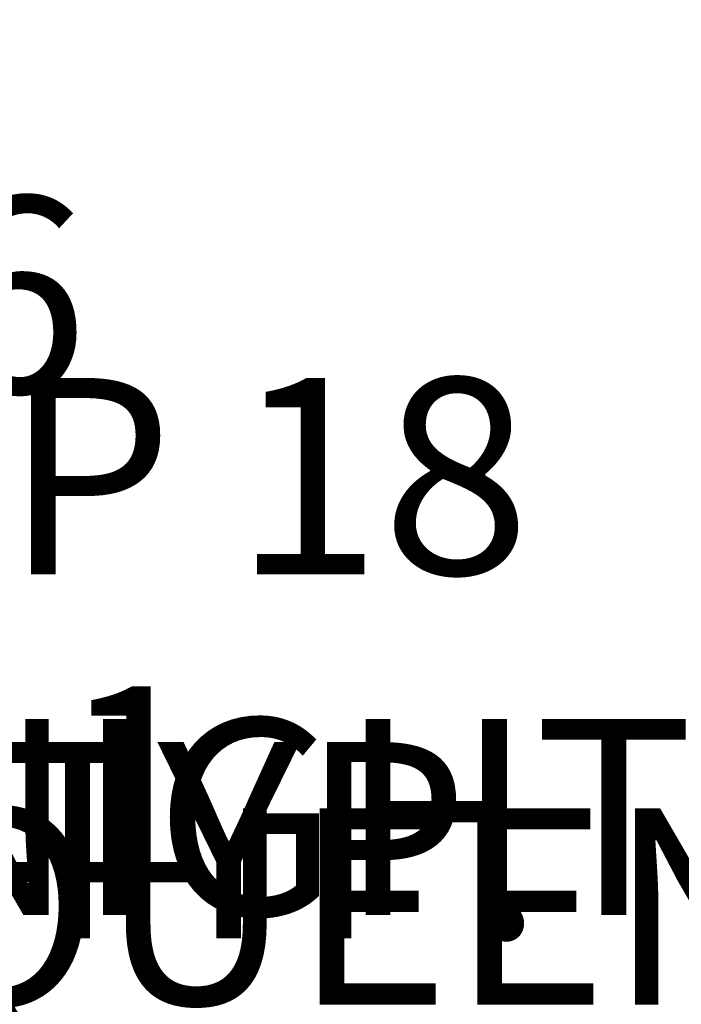
# Model space of a CAD drawing. Units: inches. Extents: x 1173 to 2157, y 515 to 1129.
# Tile 12 of 13: x 1702 to 1824, y 948 to 1129. Entities that reach past the tile are written whole.
import ezdxf

# ---------------------------------------------------------------- set-up
doc = ezdxf.new("R2010")
doc.units = ezdxf.units.IN
doc.header["$MEASUREMENT"] = 0
doc.layers.add('A-ANNO-DIMS', color=2, linetype='Continuous', lineweight=18)
doc.styles.get("Standard").update_dxf_attribs({"font": 'arial.ttf'})
doc.dimstyles.get("Standard").update_dxf_attribs({"dimtxt": 36, "dimasz": 0.18, "dimexe": 0.18, "dimexo": 0.0625, "dimgap": 0.09, "dimtad": 0, "dimtih": 1, "dimtoh": 1, "dimdec": 0, "dimrnd": 72, "dimzin": 0, "dimdsep": 46, "dimlunit": 3, "dimtxsty": 'Standard', "dimcen": 2, "dimadec": 0, "dimazin": 0, "dimtfac": 1, "dimtdec": 0, "dimtofl": 0, "dimtmove": 0, "dimatfit": 3, "dimfxl": 1, "dimtolj": 1, "dimtzin": 0, "dimarcsym": 0})

# ---------------------------------------------------------------- blocks, each defined once
blk = doc.blocks.new('*D28')
at = {"layer": 'A-ANNO-DIMS', "color": 0, "lineweight": -2, "transparency": 16777216}
for p, q in [((1581.66, 978.31), (1581.66, 966.19)), ((1661.66, 978.31), (1661.66, 966.19)), ((1581.84, 966.37), (1661.48, 966.37)), ((1661.66, 966.37), (1661.84, 966.37))]:
    blk.add_line(p, q, dxfattribs=at)
at = {"layer": 'A-ANNO-DIMS', "color": 0, "transparency": 16777216}
for points in [[(1581.84, 966.4), (1581.84, 966.34), (1581.66, 966.37)], [(1661.48, 966.4), (1661.48, 966.34), (1661.66, 966.37)]]:
    blk.add_solid(points, dxfattribs=at)
at = {"layer": 'Defpoints', "color": 0, "transparency": 16777216}
for p in [(1581.66, 978.37), (1661.66, 978.37), (1661.66, 966.37)]:
    blk.add_point(p, dxfattribs=at)
at = {"layer": 'A-ANNO-DIMS', "color": 0, "transparency": 16777216, "insert": (1904.61, 966.37), "char_height": 36, "attachment_point": 5}
blk.add_mtext('\\A1;QUEEN BED 80 TYP.', dxfattribs=at)
blk = doc.blocks.new('*D34')
at = {"layer": 'A-ANNO-DIMS', "color": 0, "lineweight": -2, "transparency": 16777216}
for p, q in [((1631.9, 978.41), (1631.9, 982.97)), ((1661.5, 978.41), (1661.5, 982.97)), ((1632.08, 982.79), (1661.32, 982.79)), ((1661.5, 982.79), (1661.68, 982.79))]:
    blk.add_line(p, q, dxfattribs=at)
at = {"layer": 'A-ANNO-DIMS', "color": 0, "transparency": 16777216}
for points in [[(1632.08, 982.82), (1632.08, 982.76), (1631.9, 982.79)], [(1661.32, 982.82), (1661.32, 982.76), (1661.5, 982.79)]]:
    blk.add_solid(points, dxfattribs=at)
at = {"layer": 'Defpoints', "color": 0, "transparency": 16777216}
for p in [(1661.5, 982.79), (1631.9, 978.35), (1661.5, 978.35)]:
    blk.add_point(p, dxfattribs=at)
at = {"layer": 'A-ANNO-DIMS', "color": 0, "transparency": 16777216, "insert": (1918.96, 982.79), "char_height": 36, "attachment_point": 5}
blk.add_mtext('\\A1;NIGHTSTAND 30 TYP.', dxfattribs=at)
blk = doc.blocks.new('*D35')
at = {"layer": 'A-ANNO-DIMS', "color": 0, "lineweight": -2, "transparency": 16777216}
for p, q in [((1631.84, 978.35), (1627.28, 978.35)), ((1627.46, 978.35), (1627.46, 978.53)), ((1627.46, 978.53), (1627.64, 978.53)), ((1627.46, 949.05), (1627.46, 978.17)), ((1631.84, 948.87), (1627.28, 948.87))]:
    blk.add_line(p, q, dxfattribs=at)
at = {"layer": 'A-ANNO-DIMS', "color": 0, "transparency": 16777216}
for points in [[(1627.43, 978.17), (1627.49, 978.17), (1627.46, 978.35)], [(1627.43, 949.05), (1627.49, 949.05), (1627.46, 948.87)]]:
    blk.add_solid(points, dxfattribs=at)
at = {"layer": 'Defpoints', "color": 0, "transparency": 16777216}
for p in [(1627.46, 978.35), (1631.9, 978.35), (1631.9, 948.87)]:
    blk.add_point(p, dxfattribs=at)
at = {"layer": 'A-ANNO-DIMS', "color": 0, "transparency": 16777216, "insert": (1715.66, 978.53), "char_height": 36, "attachment_point": 5}
blk.add_mtext('\\A1;29 TYP.', dxfattribs=at)
blk = doc.blocks.new('*D62')
at = {"layer": 'A-ANNO-DIMS', "color": 0, "lineweight": -2, "transparency": 16777216}
for p, q in [((1491.7, 1042.71), (1491.7, 1045.52)), ((1491.88, 1045.34), (1509.47, 1045.34)), ((1509.65, 1042.71), (1509.65, 1045.52)), ((1509.65, 1045.34), (1509.83, 1045.34))]:
    blk.add_line(p, q, dxfattribs=at)
at = {"layer": 'A-ANNO-DIMS', "color": 0, "transparency": 16777216}
for points in [[(1491.88, 1045.37), (1491.88, 1045.31), (1491.7, 1045.34)], [(1509.47, 1045.37), (1509.47, 1045.31), (1509.65, 1045.34)]]:
    blk.add_solid(points, dxfattribs=at)
at = {"layer": 'Defpoints', "color": 0, "transparency": 16777216}
for p in [(1509.65, 1045.34), (1491.7, 1042.65), (1509.65, 1042.65)]:
    blk.add_point(p, dxfattribs=at)
at = {"layer": 'A-ANNO-DIMS', "color": 0, "transparency": 16777216, "insert": (1657.22, 1045.34), "char_height": 36, "attachment_point": 5}
blk.add_mtext('\\A1;SINK TAP 18', dxfattribs=at)
blk = doc.blocks.new('*D90')
at = {"layer": 'A-ANNO-DIMS', "color": 0, "lineweight": -2, "transparency": 16777216}
for p, q in [((1661.73, 1044.28), (1696.15, 1044.28)), ((1695.97, 1044.1), (1695.97, 1006.94)), ((1695.97, 933.46), (1695.97, 970.62)), ((1625.73, 933.28), (1696.15, 933.28))]:
    blk.add_line(p, q, dxfattribs=at)
at = {"layer": 'A-ANNO-DIMS', "color": 0, "transparency": 16777216}
for points in [[(1695.94, 1044.1), (1696, 1044.1), (1695.97, 1044.28)], [(1695.94, 933.46), (1696, 933.46), (1695.97, 933.28)]]:
    blk.add_solid(points, dxfattribs=at)
at = {"layer": 'Defpoints', "color": 0, "transparency": 16777216}
for p in [(1661.66, 1044.28), (1625.66, 933.28), (1695.97, 933.28)]:
    blk.add_point(p, dxfattribs=at)
at = {"layer": 'A-ANNO-DIMS', "color": 0, "transparency": 16777216, "insert": (1695.97, 988.78), "char_height": 36, "attachment_point": 5}
blk.add_mtext('\\A1;111', dxfattribs=at)
blk = doc.blocks.new('*D98')
at = {"layer": 'A-ANNO-DIMS', "color": 0, "lineweight": -2, "transparency": 16777216}
for p, q in [((1625.66, 924.34), (1625.66, 1078.79)), ((1625.84, 1078.61), (1661.48, 1078.61)), ((1661.66, 924.34), (1661.66, 1078.79)), ((1661.66, 1078.61), (1661.84, 1078.61))]:
    blk.add_line(p, q, dxfattribs=at)
at = {"layer": 'A-ANNO-DIMS', "color": 0, "transparency": 16777216}
for points in [[(1625.84, 1078.64), (1625.84, 1078.58), (1625.66, 1078.61)], [(1661.48, 1078.64), (1661.48, 1078.58), (1661.66, 1078.61)]]:
    blk.add_solid(points, dxfattribs=at)
at = {"layer": 'Defpoints', "color": 0, "transparency": 16777216}
for p in [(1661.66, 1078.61), (1625.66, 924.28), (1661.66, 924.28)]:
    blk.add_point(p, dxfattribs=at)
at = {"layer": 'A-ANNO-DIMS', "color": 0, "transparency": 16777216, "insert": (1687.69, 1078.61), "char_height": 36, "attachment_point": 5}
blk.add_mtext('\\A1;36', dxfattribs=at)

msp = doc.modelspace()

# ---------------------------------------------------------------- dimensions: what is measured, and where the dimension line sits
at = {"layer": 'A-ANNO-DIMS'}
for base, p1, p2, text, picture, middle in [((1509.6463, 1045.3406), (1491.6951, 1042.6479), (1509.6463, 1042.6479), 'SINK TAP <>', '*D62', (1657.2192, 1045.3406)), ((1661.6635, 966.3712), (1581.6634, 978.3712), (1661.6635, 978.3712), 'QUEEN BED <> TYP.', '*D28', (1904.6142, 966.3712)), ((1661.5047, 982.7919), (1631.9047, 978.3519), (1661.5047, 978.3519), 'NIGHTSTAND <> TYP.', '*D34', (1918.9562, 982.7919))]:
    dim = msp.add_linear_dim(base=base, p1=p1, p2=p2, text=text, dimstyle='Standard', override={"dimdec": 0, "dimlfac": 1, "dimrnd": 0, "dimzin": 0, "dimdsep": 46, "dimlunit": 2}, dxfattribs=at)
    dim.commit()
    dim.dimension.update_dxf_attribs({"geometry": picture, "text_midpoint": middle})
dim = msp.add_linear_dim(base=(1661.6635, 1078.6127), p1=(1625.6635, 924.2805), p2=(1661.6635, 924.2805), dimstyle='Standard', override={"dimdec": 0, "dimlfac": 1, "dimrnd": 0, "dimzin": 0, "dimdsep": 46, "dimlunit": 2}, dxfattribs=at)
dim.commit()
dim.dimension.update_dxf_attribs({"geometry": '*D98', "text_midpoint": (1687.6933, 1078.6127)})
dim = msp.add_linear_dim(base=(1695.966, 933.2805), p1=(1661.6635, 1044.2805), p2=(1625.6635, 933.2805), angle=90, dimstyle='Standard', override={"dimdec": 0, "dimlfac": 1, "dimrnd": 0, "dimzin": 0, "dimdsep": 46, "dimlunit": 2}, dxfattribs=at)
dim.commit()
dim.dimension.update_dxf_attribs({"geometry": '*D90', "text_midpoint": (1695.966, 988.7805)})
dim = msp.add_linear_dim(base=(1627.4647, 978.3519), p1=(1631.9047, 948.8672), p2=(1631.9047, 978.3519), angle=90, text='<> TYP.', dimstyle='Standard', override={"dimdec": 0, "dimlfac": 1, "dimrnd": 0, "dimzin": 0, "dimdsep": 46, "dimlunit": 2}, dxfattribs=at)
dim.commit()
dim.dimension.update_dxf_attribs({"geometry": '*D35', "text_midpoint": (1715.6597, 978.5319)})

doc.saveas('drawing.dxf')
